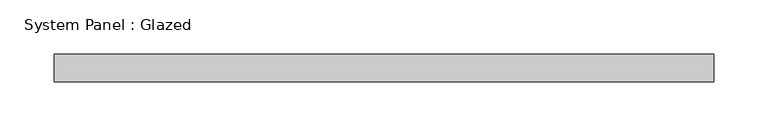
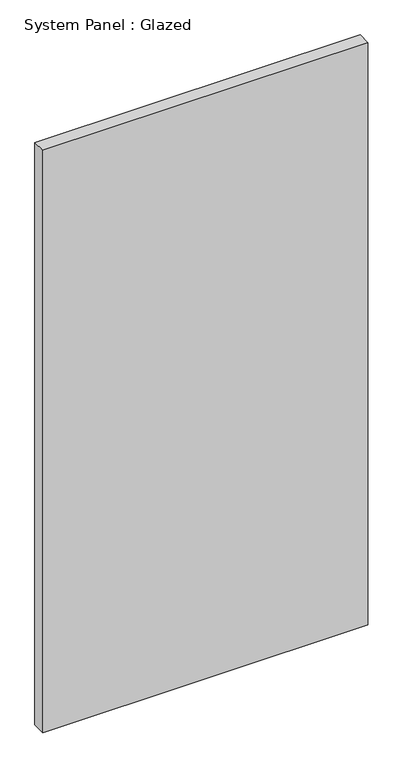
"""IFC4 building model written with IfcOpenShell, lengths in millimetres: plate geometry, System Panel : Glazed."""

from ifc_helpers import new_model, si_unit, origin, origin_with_axes, place, context, project, spatial, polyline, outline, extrude, source, transform, mapped, element, save


def system_panel_glazed_188537b2(model_context):
    return source(origin(), model_context, "Body", "SweptSolid", [
        extrude(outline(polyline([(305.0132811, 19.05), (-305.0132811, 19.05), (-305.0132811, 44.45), (305.0132811, 44.45), (305.0132811, 19.05)])), origin_with_axes(), (0.0, 0.0, 1.0), 1155.7),
    ])


if __name__ == "__main__":
    model = new_model("IFC4")
    model_context = context("Model", 3, world=origin())
    ifc_project = project(units=[si_unit("LENGTHUNIT", "METRE", prefix="MILLI")], contexts=[model_context])
    site = spatial("IfcSite", under=ifc_project)
    building = spatial("IfcBuilding", under=site)
    placement = place(None, origin())
    system_panel_glazed_shape = system_panel_glazed_188537b2(model_context)
    element("IfcPlate", 1, ObjectType="System Panel : Glazed", at=placement, inside=building, context=model_context, shape_type="MappedRepresentation", body=[
        mapped(system_panel_glazed_shape, transform((0.0, 0.0, 0.0), x_axis=(1.0, 0.0, 0.0), y_axis=(0.0, 1.0, 0.0), z_axis=(0.0, 0.0, 1.0))),
    ])
    save(model, "model.ifc")

# Revit data of these elements
# Type "System Panel : Glazed"
#   Construction Type Id = "GSP4R"
#   Analytic Construction = "1/8 in Pilkington single glazing"
#   Visual Light Transmittance = 0.9
#   Solar Heat Gain Coefficient = 0.86
#   Heat Transfer Coefficient (U) = 1.18115 BTU/(h·ft²·°F)
# Element 1 (IfcPlate, "System Panel : Glazed")
#   Materials on its faces: "Glass"
# Materials
#   "Glass": class "Glass", colour RGB 0 128 192, transparency 0.75, Description = "Soda Lime Glass", Cost = 0
